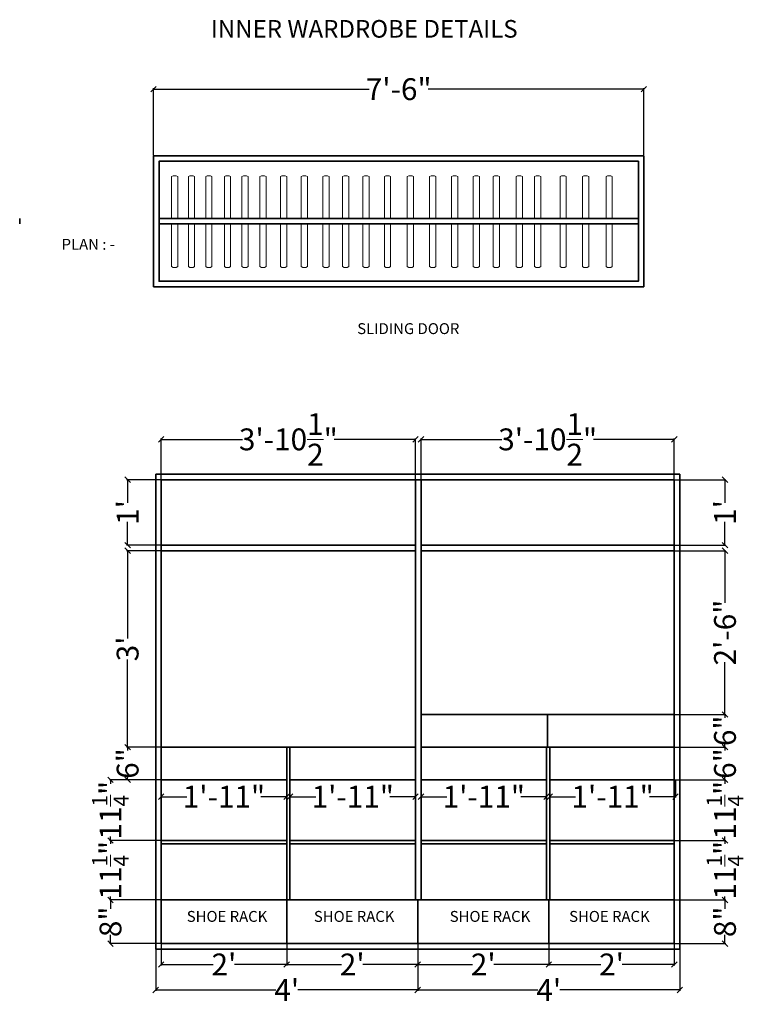
# Model space of a CAD drawing. Units: inches. Extents: x 314 to 446, y 231 to 411.
import ezdxf

# ---------------------------------------------------------------- set-up
doc = ezdxf.new("R2010")
doc.units = ezdxf.units.IN
doc.header["$MEASUREMENT"] = 0
for name, color, linetype, lineweight in [('A-ANNO-DIMS', 2, 'Continuous', 18), ('A-ANNO-TEXT', 7, 'Continuous', 25), ('A-FURN', 7, 'Continuous', 35), ('A-FURN-HANG', 8, 'Continuous', 18)]:
    doc.layers.add(name, color=color, linetype=linetype, lineweight=lineweight)
doc.styles.get("Standard").update_dxf_attribs({"font": 'arial.ttf'})
doc.dimstyles.get("Standard").update_dxf_attribs({"dimtxt": 4, "dimasz": 1, "dimexe": 0.18, "dimexo": 0.0625, "dimgap": 0.09, "dimtad": 0, "dimdec": 1, "dimzin": 0, "dimdsep": 46, "dimlunit": 4, "dimtxsty": 'Standard', "dimblk": 'OBLIQUE', "dimcen": 0.09, "dimadec": 0, "dimazin": 0, "dimtfac": 1, "dimtdec": 1, "dimtofl": 0, "dimtmove": 0, "dimatfit": 3, "dimldrblk": 'OBLIQUE', "dimfxl": 1, "dimtolj": 1, "dimtzin": 0, "dimarcsym": 1})

# ---------------------------------------------------------------- blocks, each defined once
blk = doc.blocks.new('_Oblique')
at = {"color": 0, "linetype": 'ByBlock', "lineweight": -2}
blk.add_line((-0.5, -0.5), (0.5, 0.5), dxfattribs=at)
blk = doc.blocks.new('*D2')
at = {"layer": 'A-ANNO-DIMS', "color": 0, "lineweight": -2, "transparency": 16777216}
for p, q in [((338.41, 386.23), (338.41, 398.53)), ((338.41, 398.35), (377.92, 398.35)), ((428.21, 398.35), (388.7, 398.35)), ((428.21, 386.23), (428.21, 398.53))]:
    blk.add_line(p, q, dxfattribs=at)
at = {"layer": 'Defpoints', "color": 0, "transparency": 16777216}
for p in [(428.21, 398.35), (338.41, 386.16), (428.21, 386.16)]:
    blk.add_point(p, dxfattribs=at)
at = {"layer": 'A-ANNO-DIMS', "color": 0, "lineweight": -2, "transparency": 16777216, "rotation": 180}
blk.add_blockref('_Oblique', (338.41, 398.35), dxfattribs=at)
at = {"layer": 'A-ANNO-DIMS', "color": 0, "lineweight": -2, "transparency": 16777216}
blk.add_blockref('_Oblique', (428.21, 398.35), dxfattribs=at)
at = {"layer": 'A-ANNO-DIMS', "color": 0, "transparency": 16777216, "insert": (383.31, 398.35), "char_height": 4, "width": 10.6003, "attachment_point": 5}
blk.add_mtext('\\A1;7\'-6"', dxfattribs=at)
blk = doc.blocks.new('*D3')
at = {"layer": 'A-ANNO-DIMS', "color": 0, "lineweight": -2, "transparency": 16777216}
for p, q in [((339.8, 271.74), (339.8, 268.55)), ((362.8, 271.74), (362.8, 268.55)), ((339.8, 268.73), (344.52, 268.73)), ((362.8, 268.73), (358.07, 268.73))]:
    blk.add_line(p, q, dxfattribs=at)
at = {"layer": 'Defpoints', "color": 0, "transparency": 16777216}
for p in [(339.8, 271.8), (362.8, 271.8), (339.8, 268.73)]:
    blk.add_point(p, dxfattribs=at)
at = {"layer": 'A-ANNO-DIMS', "color": 0, "lineweight": -2, "transparency": 16777216, "rotation": 180}
blk.add_blockref('_Oblique', (339.8, 268.73), dxfattribs=at)
at = {"layer": 'A-ANNO-DIMS', "color": 0, "lineweight": -2, "transparency": 16777216}
blk.add_blockref('_Oblique', (362.8, 268.73), dxfattribs=at)
at = {"layer": 'A-ANNO-DIMS', "color": 0, "transparency": 16777216, "insert": (351.3, 268.73), "char_height": 4, "attachment_point": 5}
blk.add_mtext('\\A1;1\'-11"', dxfattribs=at)
blk = doc.blocks.new('*D4')
at = {"layer": 'A-ANNO-DIMS', "color": 0, "lineweight": -2, "transparency": 16777216}
for p, q in [((363.4, 271.74), (363.4, 268.55)), ((386.4, 271.74), (386.4, 268.55)), ((363.4, 268.73), (368.12, 268.73)), ((386.4, 268.73), (381.67, 268.73))]:
    blk.add_line(p, q, dxfattribs=at)
at = {"layer": 'Defpoints', "color": 0, "transparency": 16777216}
for p in [(363.4, 271.8), (386.4, 271.8), (386.4, 268.73)]:
    blk.add_point(p, dxfattribs=at)
at = {"layer": 'A-ANNO-DIMS', "color": 0, "lineweight": -2, "transparency": 16777216, "rotation": 180}
blk.add_blockref('_Oblique', (363.4, 268.73), dxfattribs=at)
at = {"layer": 'A-ANNO-DIMS', "color": 0, "lineweight": -2, "transparency": 16777216}
blk.add_blockref('_Oblique', (386.4, 268.73), dxfattribs=at)
at = {"layer": 'A-ANNO-DIMS', "color": 0, "transparency": 16777216, "insert": (374.9, 268.73), "char_height": 4, "attachment_point": 5}
blk.add_mtext('\\A1;1\'-11"', dxfattribs=at)
blk = doc.blocks.new('*D5')
at = {"layer": 'A-ANNO-DIMS', "color": 0, "lineweight": -2, "transparency": 16777216}
for p, q in [((339.8, 241.74), (339.8, 237.81)), ((362.8, 241.74), (362.8, 237.81)), ((339.8, 237.99), (349.33, 237.99)), ((362.8, 237.99), (353.26, 237.99))]:
    blk.add_line(p, q, dxfattribs=at)
at = {"layer": 'Defpoints', "color": 0, "transparency": 16777216}
for p in [(339.8, 241.8), (362.8, 241.8), (362.8, 237.99)]:
    blk.add_point(p, dxfattribs=at)
at = {"layer": 'A-ANNO-DIMS', "color": 0, "lineweight": -2, "transparency": 16777216, "rotation": 180}
blk.add_blockref('_Oblique', (339.8, 237.99), dxfattribs=at)
at = {"layer": 'A-ANNO-DIMS', "color": 0, "lineweight": -2, "transparency": 16777216}
blk.add_blockref('_Oblique', (362.8, 237.99), dxfattribs=at)
at = {"layer": 'A-ANNO-DIMS', "color": 0, "transparency": 16777216, "insert": (351.3, 237.99), "char_height": 4, "attachment_point": 5}
blk.add_mtext("\\A1;2'", dxfattribs=at)
blk = doc.blocks.new('*D6')
at = {"layer": 'A-ANNO-DIMS', "color": 0, "lineweight": -2, "transparency": 16777216}
for p, q in [((362.8, 241.74), (362.8, 237.81)), ((386.8, 241.74), (386.8, 237.81)), ((362.8, 237.99), (372.83, 237.99)), ((386.8, 237.99), (376.76, 237.99))]:
    blk.add_line(p, q, dxfattribs=at)
at = {"layer": 'Defpoints', "color": 0, "transparency": 16777216}
for p in [(362.8, 241.8), (386.8, 241.8), (386.8, 237.99)]:
    blk.add_point(p, dxfattribs=at)
at = {"layer": 'A-ANNO-DIMS', "color": 0, "lineweight": -2, "transparency": 16777216, "rotation": 180}
blk.add_blockref('_Oblique', (362.8, 237.99), dxfattribs=at)
at = {"layer": 'A-ANNO-DIMS', "color": 0, "lineweight": -2, "transparency": 16777216}
blk.add_blockref('_Oblique', (386.8, 237.99), dxfattribs=at)
at = {"layer": 'A-ANNO-DIMS', "color": 0, "transparency": 16777216, "insert": (374.8, 237.99), "char_height": 4, "attachment_point": 5}
blk.add_mtext("\\A1;2'", dxfattribs=at)
blk = doc.blocks.new('*D7')
at = {"layer": 'A-ANNO-DIMS', "color": 0, "lineweight": -2, "transparency": 16777216}
for p, q in [((386.8, 241.74), (386.8, 237.81)), ((410.8, 241.74), (410.8, 237.81)), ((386.8, 237.99), (396.83, 237.99)), ((410.8, 237.99), (400.76, 237.99))]:
    blk.add_line(p, q, dxfattribs=at)
at = {"layer": 'Defpoints', "color": 0, "transparency": 16777216}
for p in [(386.8, 241.8), (410.8, 241.8), (410.8, 237.99)]:
    blk.add_point(p, dxfattribs=at)
at = {"layer": 'A-ANNO-DIMS', "color": 0, "lineweight": -2, "transparency": 16777216, "rotation": 180}
blk.add_blockref('_Oblique', (386.8, 237.99), dxfattribs=at)
at = {"layer": 'A-ANNO-DIMS', "color": 0, "lineweight": -2, "transparency": 16777216}
blk.add_blockref('_Oblique', (410.8, 237.99), dxfattribs=at)
at = {"layer": 'A-ANNO-DIMS', "color": 0, "transparency": 16777216, "insert": (398.8, 237.99), "char_height": 4, "attachment_point": 5}
blk.add_mtext("\\A1;2'", dxfattribs=at)
blk = doc.blocks.new('*D8')
at = {"layer": 'A-ANNO-DIMS', "color": 0, "lineweight": -2, "transparency": 16777216}
for p, q in [((410.8, 241.74), (410.8, 237.81)), ((433.8, 241.74), (433.8, 237.81)), ((410.8, 237.99), (420.33, 237.99)), ((433.8, 237.99), (424.26, 237.99))]:
    blk.add_line(p, q, dxfattribs=at)
at = {"layer": 'Defpoints', "color": 0, "transparency": 16777216}
for p in [(410.8, 241.8), (433.8, 241.8), (410.8, 237.99)]:
    blk.add_point(p, dxfattribs=at)
at = {"layer": 'A-ANNO-DIMS', "color": 0, "lineweight": -2, "transparency": 16777216, "rotation": 180}
blk.add_blockref('_Oblique', (410.8, 237.99), dxfattribs=at)
at = {"layer": 'A-ANNO-DIMS', "color": 0, "lineweight": -2, "transparency": 16777216}
blk.add_blockref('_Oblique', (433.8, 237.99), dxfattribs=at)
at = {"layer": 'A-ANNO-DIMS', "color": 0, "transparency": 16777216, "insert": (422.3, 237.99), "char_height": 4, "attachment_point": 5}
blk.add_mtext("\\A1;2'", dxfattribs=at)
blk = doc.blocks.new('*D9')
at = {"layer": 'A-ANNO-DIMS', "color": 0, "lineweight": -2, "transparency": 16777216}
for p, q in [((338.8, 240.74), (338.8, 233.13)), ((386.8, 240.74), (386.8, 233.13)), ((338.8, 233.31), (360.79, 233.31)), ((386.8, 233.31), (364.81, 233.31))]:
    blk.add_line(p, q, dxfattribs=at)
at = {"layer": 'Defpoints', "color": 0, "transparency": 16777216}
for p in [(338.8, 240.8), (386.8, 240.8), (386.8, 233.31)]:
    blk.add_point(p, dxfattribs=at)
at = {"layer": 'A-ANNO-DIMS', "color": 0, "lineweight": -2, "transparency": 16777216, "rotation": 180}
blk.add_blockref('_Oblique', (338.8, 233.31), dxfattribs=at)
at = {"layer": 'A-ANNO-DIMS', "color": 0, "lineweight": -2, "transparency": 16777216}
blk.add_blockref('_Oblique', (386.8, 233.31), dxfattribs=at)
at = {"layer": 'A-ANNO-DIMS', "color": 0, "transparency": 16777216, "insert": (362.8, 233.31), "char_height": 4, "attachment_point": 5}
blk.add_mtext("\\A1;4'", dxfattribs=at)
blk = doc.blocks.new('*D10')
at = {"layer": 'A-ANNO-DIMS', "color": 0, "lineweight": -2, "transparency": 16777216}
for p, q in [((386.8, 240.74), (386.8, 233.13)), ((434.8, 240.74), (434.8, 233.13)), ((386.8, 233.31), (408.79, 233.31)), ((434.8, 233.31), (412.81, 233.31))]:
    blk.add_line(p, q, dxfattribs=at)
at = {"layer": 'Defpoints', "color": 0, "transparency": 16777216}
for p in [(386.8, 240.8), (434.8, 240.8), (434.8, 233.31)]:
    blk.add_point(p, dxfattribs=at)
at = {"layer": 'A-ANNO-DIMS', "color": 0, "lineweight": -2, "transparency": 16777216, "rotation": 180}
blk.add_blockref('_Oblique', (386.8, 233.31), dxfattribs=at)
at = {"layer": 'A-ANNO-DIMS', "color": 0, "lineweight": -2, "transparency": 16777216}
blk.add_blockref('_Oblique', (434.8, 233.31), dxfattribs=at)
at = {"layer": 'A-ANNO-DIMS', "color": 0, "transparency": 16777216, "insert": (410.8, 233.31), "char_height": 4, "attachment_point": 5}
blk.add_mtext("\\A1;4'", dxfattribs=at)
blk = doc.blocks.new('*D11')
at = {"layer": 'A-ANNO-DIMS', "color": 0, "lineweight": -2, "transparency": 16777216}
for p, q in [((387.4, 271.74), (387.4, 268.55)), ((410.4, 271.74), (410.4, 268.55)), ((387.4, 268.73), (392.12, 268.73)), ((410.4, 268.73), (405.67, 268.73))]:
    blk.add_line(p, q, dxfattribs=at)
at = {"layer": 'Defpoints', "color": 0, "transparency": 16777216}
for p in [(387.4, 271.8), (410.4, 271.8), (387.4, 268.73)]:
    blk.add_point(p, dxfattribs=at)
at = {"layer": 'A-ANNO-DIMS', "color": 0, "lineweight": -2, "transparency": 16777216, "rotation": 180}
blk.add_blockref('_Oblique', (387.4, 268.73), dxfattribs=at)
at = {"layer": 'A-ANNO-DIMS', "color": 0, "lineweight": -2, "transparency": 16777216}
blk.add_blockref('_Oblique', (410.4, 268.73), dxfattribs=at)
at = {"layer": 'A-ANNO-DIMS', "color": 0, "transparency": 16777216, "insert": (398.9, 268.73), "char_height": 4, "attachment_point": 5}
blk.add_mtext('\\A1;1\'-11"', dxfattribs=at)
blk = doc.blocks.new('*D12')
at = {"layer": 'A-ANNO-DIMS', "color": 0, "lineweight": -2, "transparency": 16777216}
for p, q in [((411, 271.74), (411, 268.55)), ((434, 271.74), (434, 268.55)), ((411, 268.73), (415.72, 268.73)), ((434, 268.73), (429.27, 268.73))]:
    blk.add_line(p, q, dxfattribs=at)
at = {"layer": 'Defpoints', "color": 0, "transparency": 16777216}
for p in [(411, 271.8), (434, 271.8), (434, 268.73)]:
    blk.add_point(p, dxfattribs=at)
at = {"layer": 'A-ANNO-DIMS', "color": 0, "lineweight": -2, "transparency": 16777216, "rotation": 180}
blk.add_blockref('_Oblique', (411, 268.73), dxfattribs=at)
at = {"layer": 'A-ANNO-DIMS', "color": 0, "lineweight": -2, "transparency": 16777216}
blk.add_blockref('_Oblique', (434, 268.73), dxfattribs=at)
at = {"layer": 'A-ANNO-DIMS', "color": 0, "transparency": 16777216, "insert": (422.5, 268.73), "char_height": 4, "attachment_point": 5}
blk.add_mtext('\\A1;1\'-11"', dxfattribs=at)
blk = doc.blocks.new('*D13')
at = {"layer": 'A-ANNO-DIMS', "color": 0, "lineweight": -2, "transparency": 16777216}
for p, q in [((339.8, 326.86), (339.8, 334.37)), ((339.8, 334.19), (354.68, 334.19)), ((386.4, 334.19), (371.51, 334.19)), ((386.4, 326.86), (386.4, 334.37))]:
    blk.add_line(p, q, dxfattribs=at)
at = {"layer": 'Defpoints', "color": 0, "transparency": 16777216}
for p in [(386.4, 334.19), (339.8, 326.8), (386.4, 326.8)]:
    blk.add_point(p, dxfattribs=at)
at = {"layer": 'A-ANNO-DIMS', "color": 0, "lineweight": -2, "transparency": 16777216, "rotation": 180}
blk.add_blockref('_Oblique', (339.8, 334.19), dxfattribs=at)
at = {"layer": 'A-ANNO-DIMS', "color": 0, "lineweight": -2, "transparency": 16777216}
blk.add_blockref('_Oblique', (386.4, 334.19), dxfattribs=at)
at = {"layer": 'A-ANNO-DIMS', "color": 0, "transparency": 16777216, "insert": (363.1, 334.19), "char_height": 4, "attachment_point": 5}
blk.add_mtext('\\A1;3\'-10{\\H1x;\\S1/2;}"', dxfattribs=at)
blk = doc.blocks.new('*D14')
at = {"layer": 'A-ANNO-DIMS', "color": 0, "lineweight": -2, "transparency": 16777216}
for p, q in [((387.4, 326.86), (387.4, 334.37)), ((387.4, 334.19), (402.18, 334.19)), ((433.8, 334.19), (419.01, 334.19)), ((433.8, 326.86), (433.8, 334.37))]:
    blk.add_line(p, q, dxfattribs=at)
at = {"layer": 'Defpoints', "color": 0, "transparency": 16777216}
for p in [(433.8, 334.19), (387.4, 326.8), (433.8, 326.8)]:
    blk.add_point(p, dxfattribs=at)
at = {"layer": 'A-ANNO-DIMS', "color": 0, "lineweight": -2, "transparency": 16777216, "rotation": 180}
blk.add_blockref('_Oblique', (387.4, 334.19), dxfattribs=at)
at = {"layer": 'A-ANNO-DIMS', "color": 0, "lineweight": -2, "transparency": 16777216}
blk.add_blockref('_Oblique', (433.8, 334.19), dxfattribs=at)
at = {"layer": 'A-ANNO-DIMS', "color": 0, "transparency": 16777216, "insert": (410.6, 334.19), "char_height": 4, "attachment_point": 5}
blk.add_mtext('\\A1;3\'-10{\\H1x;\\S1/2;}"', dxfattribs=at)
blk = doc.blocks.new('*D15')
at = {"layer": 'A-ANNO-DIMS', "color": 0, "lineweight": -2, "transparency": 16777216}
for p, q in [((433.86, 326.8), (443.26, 326.8)), ((443.08, 326.8), (443.08, 322.54)), ((443.08, 314.8), (443.08, 319.06)), ((433.86, 314.8), (443.26, 314.8))]:
    blk.add_line(p, q, dxfattribs=at)
at = {"layer": 'Defpoints', "color": 0, "transparency": 16777216}
for p in [(433.8, 326.8), (433.8, 314.8), (443.08, 314.8)]:
    blk.add_point(p, dxfattribs=at)
at = {"layer": 'A-ANNO-DIMS', "color": 0, "lineweight": -2, "transparency": 16777216}
for p, rotation in [((443.08, 326.8), 90), ((443.08, 314.8), 270)]:
    blk.add_blockref('_Oblique', p, dxfattribs=dict(at, rotation=rotation))
at = {"layer": 'A-ANNO-DIMS', "color": 0, "transparency": 16777216, "insert": (443.08, 320.8), "char_height": 4, "attachment_point": 5, "rotation": 90}
blk.add_mtext("\\A1;1'", dxfattribs=at)
blk = doc.blocks.new('*D16')
at = {"layer": 'A-ANNO-DIMS', "color": 0, "lineweight": -2, "transparency": 16777216}
for p, q in [((433.86, 313.8), (443.26, 313.8)), ((443.08, 313.8), (443.08, 304.24)), ((443.08, 283.8), (443.08, 293.36)), ((433.86, 283.8), (443.26, 283.8))]:
    blk.add_line(p, q, dxfattribs=at)
at = {"layer": 'Defpoints', "color": 0, "transparency": 16777216}
for p in [(433.8, 313.8), (433.8, 283.8), (443.08, 283.8)]:
    blk.add_point(p, dxfattribs=at)
at = {"layer": 'A-ANNO-DIMS', "color": 0, "lineweight": -2, "transparency": 16777216}
for p, rotation in [((443.08, 313.8), 90), ((443.08, 283.8), 270)]:
    blk.add_blockref('_Oblique', p, dxfattribs=dict(at, rotation=rotation))
at = {"layer": 'A-ANNO-DIMS', "color": 0, "transparency": 16777216, "insert": (443.08, 298.8), "char_height": 4, "attachment_point": 5, "rotation": 90}
blk.add_mtext('\\A1;2\'-6"', dxfattribs=at)
blk = doc.blocks.new('*D17')
at = {"layer": 'A-ANNO-DIMS', "color": 0, "lineweight": -2, "transparency": 16777216}
for p, q in [((433.86, 283.8), (443.26, 283.8)), ((443.08, 283.8), (443.08, 283.2)), ((443.08, 277.8), (443.08, 278.4)), ((433.86, 277.8), (443.26, 277.8))]:
    blk.add_line(p, q, dxfattribs=at)
at = {"layer": 'Defpoints', "color": 0, "transparency": 16777216}
for p in [(433.8, 283.8), (433.8, 277.8), (443.08, 277.8)]:
    blk.add_point(p, dxfattribs=at)
at = {"layer": 'A-ANNO-DIMS', "color": 0, "lineweight": -2, "transparency": 16777216}
for p, rotation in [((443.08, 283.8), 90), ((443.08, 277.8), 270)]:
    blk.add_blockref('_Oblique', p, dxfattribs=dict(at, rotation=rotation))
at = {"layer": 'A-ANNO-DIMS', "color": 0, "transparency": 16777216, "insert": (443.08, 280.8), "char_height": 4, "attachment_point": 5, "rotation": 90}
blk.add_mtext('\\A1;6"', dxfattribs=at)
blk = doc.blocks.new('*D18')
at = {"layer": 'A-ANNO-DIMS', "color": 0, "lineweight": -2, "transparency": 16777216}
for p, q in [((433.86, 277.8), (443.26, 277.8)), ((443.08, 277.8), (443.08, 277.2)), ((443.08, 271.8), (443.08, 272.4)), ((433.86, 271.8), (443.26, 271.8))]:
    blk.add_line(p, q, dxfattribs=at)
at = {"layer": 'Defpoints', "color": 0, "transparency": 16777216}
for p in [(433.8, 277.8), (433.8, 271.8), (443.08, 271.8)]:
    blk.add_point(p, dxfattribs=at)
at = {"layer": 'A-ANNO-DIMS', "color": 0, "lineweight": -2, "transparency": 16777216}
for p, rotation in [((443.08, 277.8), 90), ((443.08, 271.8), 270)]:
    blk.add_blockref('_Oblique', p, dxfattribs=dict(at, rotation=rotation))
at = {"layer": 'A-ANNO-DIMS', "color": 0, "transparency": 16777216, "insert": (443.08, 274.8), "char_height": 4, "attachment_point": 5, "rotation": 90}
blk.add_mtext('\\A1;6"', dxfattribs=at)
blk = doc.blocks.new('*D19')
at = {"layer": 'A-ANNO-DIMS', "color": 0, "lineweight": -2, "transparency": 16777216}
for p, q in [((433.86, 271.8), (443.26, 271.8)), ((443.08, 271.8), (443.08, 271.07)), ((433.86, 260.7), (443.26, 260.7)), ((443.08, 260.7), (443.08, 261.44))]:
    blk.add_line(p, q, dxfattribs=at)
at = {"layer": 'Defpoints', "color": 0, "transparency": 16777216}
for p in [(433.8, 271.8), (433.8, 260.7), (443.08, 260.7)]:
    blk.add_point(p, dxfattribs=at)
at = {"layer": 'A-ANNO-DIMS', "color": 0, "lineweight": -2, "transparency": 16777216}
for p, rotation in [((443.08, 271.8), 90), ((443.08, 260.7), 270)]:
    blk.add_blockref('_Oblique', p, dxfattribs=dict(at, rotation=rotation))
at = {"layer": 'A-ANNO-DIMS', "color": 0, "transparency": 16777216, "insert": (443.08, 266.25), "char_height": 4, "attachment_point": 5, "rotation": 90}
blk.add_mtext('\\A1;11{\\H0.7x;\\S1/4;}"', dxfattribs=at)
blk = doc.blocks.new('*D20')
at = {"layer": 'A-ANNO-DIMS', "color": 0, "lineweight": -2, "transparency": 16777216}
for p, q in [((433.86, 260.7), (443.26, 260.7)), ((443.08, 260.7), (443.08, 260.07)), ((433.86, 249.8), (443.26, 249.8)), ((443.08, 249.8), (443.08, 250.44))]:
    blk.add_line(p, q, dxfattribs=at)
at = {"layer": 'Defpoints', "color": 0, "transparency": 16777216}
for p in [(433.8, 260.7), (433.8, 249.8), (443.08, 249.8)]:
    blk.add_point(p, dxfattribs=at)
at = {"layer": 'A-ANNO-DIMS', "color": 0, "lineweight": -2, "transparency": 16777216}
for p, rotation in [((443.08, 260.7), 90), ((443.08, 249.8), 270)]:
    blk.add_blockref('_Oblique', p, dxfattribs=dict(at, rotation=rotation))
at = {"layer": 'A-ANNO-DIMS', "color": 0, "transparency": 16777216, "insert": (443.08, 255.25), "char_height": 4, "attachment_point": 5, "rotation": 90}
blk.add_mtext('\\A1;11{\\H0.7x;\\S1/4;}"', dxfattribs=at)
blk = doc.blocks.new('*D21')
at = {"layer": 'A-ANNO-DIMS', "color": 0, "lineweight": -2, "transparency": 16777216}
for p, q in [((433.86, 249.8), (443.26, 249.8)), ((443.08, 249.8), (443.08, 248.19)), ((433.86, 241.8), (443.26, 241.8)), ((443.08, 241.8), (443.08, 243.41))]:
    blk.add_line(p, q, dxfattribs=at)
at = {"layer": 'Defpoints', "color": 0, "transparency": 16777216}
for p in [(433.8, 249.8), (433.8, 241.8), (443.08, 241.8)]:
    blk.add_point(p, dxfattribs=at)
at = {"layer": 'A-ANNO-DIMS', "color": 0, "lineweight": -2, "transparency": 16777216}
for p, rotation in [((443.08, 249.8), 90), ((443.08, 241.8), 270)]:
    blk.add_blockref('_Oblique', p, dxfattribs=dict(at, rotation=rotation))
at = {"layer": 'A-ANNO-DIMS', "color": 0, "transparency": 16777216, "insert": (443.08, 245.8), "char_height": 4, "attachment_point": 5, "rotation": 90}
blk.add_mtext('\\A1;8"', dxfattribs=at)
blk = doc.blocks.new('*D22')
at = {"layer": 'A-ANNO-DIMS', "color": 0, "lineweight": -2, "transparency": 16777216}
for p, q in [((339.73, 313.8), (333.48, 313.8)), ((333.66, 313.8), (333.66, 297.73)), ((333.66, 277.8), (333.66, 293.87)), ((339.73, 277.8), (333.48, 277.8))]:
    blk.add_line(p, q, dxfattribs=at)
at = {"layer": 'Defpoints', "color": 0, "transparency": 16777216}
for p in [(339.8, 313.8), (333.66, 277.8), (339.8, 277.8)]:
    blk.add_point(p, dxfattribs=at)
at = {"layer": 'A-ANNO-DIMS', "color": 0, "lineweight": -2, "transparency": 16777216}
for p, rotation in [((333.66, 313.8), 90), ((333.66, 277.8), 270)]:
    blk.add_blockref('_Oblique', p, dxfattribs=dict(at, rotation=rotation))
at = {"layer": 'A-ANNO-DIMS', "color": 0, "transparency": 16777216, "insert": (333.66, 295.8), "char_height": 4, "attachment_point": 5, "rotation": 90}
blk.add_mtext("\\A1;3'", dxfattribs=at)
blk = doc.blocks.new('*D23')
at = {"layer": 'A-ANNO-DIMS', "color": 0, "lineweight": -2, "transparency": 16777216}
for p, q in [((339.73, 326.8), (333.48, 326.8)), ((333.66, 326.8), (333.66, 322.54)), ((333.66, 314.8), (333.66, 319.06)), ((339.73, 314.8), (333.48, 314.8))]:
    blk.add_line(p, q, dxfattribs=at)
at = {"layer": 'Defpoints', "color": 0, "transparency": 16777216}
for p in [(339.8, 326.8), (333.66, 314.8), (339.8, 314.8)]:
    blk.add_point(p, dxfattribs=at)
at = {"layer": 'A-ANNO-DIMS', "color": 0, "lineweight": -2, "transparency": 16777216}
for p, rotation in [((333.66, 326.8), 90), ((333.66, 314.8), 270)]:
    blk.add_blockref('_Oblique', p, dxfattribs=dict(at, rotation=rotation))
at = {"layer": 'A-ANNO-DIMS', "color": 0, "transparency": 16777216, "insert": (333.66, 320.8), "char_height": 4, "attachment_point": 5, "rotation": 90}
blk.add_mtext("\\A1;1'", dxfattribs=at)
blk = doc.blocks.new('*D24')
at = {"layer": 'A-ANNO-DIMS', "color": 0, "lineweight": -2, "transparency": 16777216}
for p, q in [((339.73, 277.8), (333.48, 277.8)), ((333.66, 277.8), (333.66, 277.2)), ((333.66, 271.8), (333.66, 272.4)), ((339.73, 271.8), (333.48, 271.8))]:
    blk.add_line(p, q, dxfattribs=at)
at = {"layer": 'Defpoints', "color": 0, "transparency": 16777216}
for p in [(339.8, 277.8), (333.66, 271.8), (339.8, 271.8)]:
    blk.add_point(p, dxfattribs=at)
at = {"layer": 'A-ANNO-DIMS', "color": 0, "lineweight": -2, "transparency": 16777216}
for p, rotation in [((333.66, 277.8), 90), ((333.66, 271.8), 270)]:
    blk.add_blockref('_Oblique', p, dxfattribs=dict(at, rotation=rotation))
at = {"layer": 'A-ANNO-DIMS', "color": 0, "transparency": 16777216, "insert": (333.66, 274.8), "char_height": 4, "attachment_point": 5, "rotation": 90}
blk.add_mtext('\\A1;6"', dxfattribs=at)
blk = doc.blocks.new('*D25')
at = {"layer": 'A-ANNO-DIMS', "color": 0, "lineweight": -2, "transparency": 16777216}
for p, q in [((339.73, 271.8), (330.34, 271.8)), ((330.52, 271.8), (330.52, 271.07)), ((339.73, 260.7), (330.34, 260.7)), ((330.52, 260.7), (330.52, 261.44))]:
    blk.add_line(p, q, dxfattribs=at)
at = {"layer": 'Defpoints', "color": 0, "transparency": 16777216}
for p in [(339.8, 271.8), (330.52, 260.7), (339.8, 260.7)]:
    blk.add_point(p, dxfattribs=at)
at = {"layer": 'A-ANNO-DIMS', "color": 0, "lineweight": -2, "transparency": 16777216}
for p, rotation in [((330.52, 271.8), 90), ((330.52, 260.7), 270)]:
    blk.add_blockref('_Oblique', p, dxfattribs=dict(at, rotation=rotation))
at = {"layer": 'A-ANNO-DIMS', "color": 0, "transparency": 16777216, "insert": (330.52, 266.25), "char_height": 4, "attachment_point": 5, "rotation": 90}
blk.add_mtext('\\A1;11{\\H0.7x;\\S1/4;}"', dxfattribs=at)
blk = doc.blocks.new('*D26')
at = {"layer": 'A-ANNO-DIMS', "color": 0, "lineweight": -2, "transparency": 16777216}
for p, q in [((339.73, 260.7), (330.34, 260.7)), ((330.52, 260.7), (330.52, 260.07)), ((339.73, 249.8), (330.34, 249.8)), ((330.52, 249.8), (330.52, 250.44))]:
    blk.add_line(p, q, dxfattribs=at)
at = {"layer": 'Defpoints', "color": 0, "transparency": 16777216}
for p in [(339.8, 260.7), (330.52, 249.8), (339.8, 249.8)]:
    blk.add_point(p, dxfattribs=at)
at = {"layer": 'A-ANNO-DIMS', "color": 0, "lineweight": -2, "transparency": 16777216}
for p, rotation in [((330.52, 260.7), 90), ((330.52, 249.8), 270)]:
    blk.add_blockref('_Oblique', p, dxfattribs=dict(at, rotation=rotation))
at = {"layer": 'A-ANNO-DIMS', "color": 0, "transparency": 16777216, "insert": (330.52, 255.25), "char_height": 4, "attachment_point": 5, "rotation": 90}
blk.add_mtext('\\A1;11{\\H0.7x;\\S1/4;}"', dxfattribs=at)
blk = doc.blocks.new('*D27')
at = {"layer": 'A-ANNO-DIMS', "color": 0, "lineweight": -2, "transparency": 16777216}
for p, q in [((339.73, 249.8), (330.34, 249.8)), ((330.52, 249.8), (330.52, 248.19)), ((339.73, 241.8), (330.34, 241.8)), ((330.52, 241.8), (330.52, 243.41))]:
    blk.add_line(p, q, dxfattribs=at)
at = {"layer": 'Defpoints', "color": 0, "transparency": 16777216}
for p in [(339.8, 249.8), (330.52, 241.8), (339.8, 241.8)]:
    blk.add_point(p, dxfattribs=at)
at = {"layer": 'A-ANNO-DIMS', "color": 0, "lineweight": -2, "transparency": 16777216}
for p, rotation in [((330.52, 249.8), 90), ((330.52, 241.8), 270)]:
    blk.add_blockref('_Oblique', p, dxfattribs=dict(at, rotation=rotation))
at = {"layer": 'A-ANNO-DIMS', "color": 0, "transparency": 16777216, "insert": (330.52, 245.8), "char_height": 4, "attachment_point": 5, "rotation": 90}
blk.add_mtext('\\A1;8"', dxfattribs=at)
blk = doc.blocks.new('HANGER-A')
for points in [[(0, 0), (0, 7.66)], [(1.14, 7.66), (1.14, 0)]]:
    blk.add_lwpolyline(points)
blk.add_arc((0.57, 6.82), 1.01, 55.7557, 124.2443)
blk = doc.blocks.new('HANGER-B')
for points in [[(0, 0.18), (0, 0.18), (0, 8.01)], [(1.14, 8.01), (1.14, 0.18)]]:
    blk.add_lwpolyline(points)
blk.add_arc((0.57, 1.01), 1.01, 235.7557, 304.2443)
blk = doc.blocks.new('HANGER-C')
for points in [[(0, 0.18), (0, 8.01)], [(1.14, 8.01), (1.14, 0.18)]]:
    blk.add_lwpolyline(points)
blk.add_arc((0.57, 1.01), 1.01, 235.7557, 304.2443)

msp = doc.modelspace()

# ---------------------------------------------------------------- linework, layer by layer
at = {"layer": 'A-FURN'}
for p, q in [((313.89, 373.66), (313.89, 374.66)), ((339.41, 374.66), (427.21, 374.66)), ((427.21, 373.66), (339.41, 373.66)), ((338.8, 240.8), (338.8, 327.8)), ((338.8, 327.8), (434.8, 327.8)), ((339.8, 241.8), (339.8, 326.8)), ((339.8, 326.8), (433.8, 326.8)), ((386.4, 326.8), (386.4, 249.8)), ((387.4, 249.8), (387.4, 326.8)), ((433.8, 326.8), (433.8, 241.8)), ((434.8, 327.8), (434.8, 240.8)), ((339.8, 314.8), (386.4, 314.8)), ((387.4, 314.8), (433.8, 314.8)), ((339.8, 313.8), (386.4, 313.8)), ((387.4, 313.8), (433.8, 313.8)), ((387.4, 283.8), (433.8, 283.8)), ((410.6, 283.8), (410.6, 277.8)), ((339.8, 277.8), (386.4, 277.8)), ((362.8, 277.8), (362.8, 249.8)), ((363.4, 249.8), (363.4, 277.8)), ((387.4, 277.8), (433.8, 277.8)), ((410.4, 277.8), (410.4, 249.8)), ((411, 249.8), (411, 277.8)), ((339.8, 271.8), (362.8, 271.8)), ((363.4, 271.8), (386.4, 271.8)), ((387.4, 271.8), (410.4, 271.8)), ((411, 271.8), (433.8, 271.8)), ((339.8, 260.7), (362.8, 260.7)), ((339.8, 260.1), (362.8, 260.1)), ((363.4, 260.7), (386.4, 260.7)), ((363.4, 260.1), (386.4, 260.1)), ((387.4, 260.7), (410.4, 260.7)), ((387.4, 260.1), (410.4, 260.1)), ((411, 260.7), (433.8, 260.7)), ((411, 260.1), (433.8, 260.1)), ((433.8, 249.8), (339.8, 249.8)), ((362.8, 249.8), (362.8, 241.8)), ((386.8, 249.8), (386.8, 241.8)), ((410.8, 249.8), (410.8, 241.8)), ((433.8, 241.8), (339.8, 241.8)), ((434.8, 240.8), (338.8, 240.8))]:
    msp.add_line(p, q, dxfattribs=at)
for points in [[(428.21, 386.16), (428.21, 362.16), (338.41, 362.16), (338.41, 386.16)], [(427.21, 385.16), (427.21, 363.16), (339.41, 363.16), (339.41, 385.16)]]:
    msp.add_lwpolyline(points, close=True, dxfattribs=at)

# ---------------------------------------------------------------- block references
at = {"layer": 'A-FURN-HANG'}
for name, p in [('HANGER-A', (341.71, 374.67)), ('HANGER-A', (344.8, 374.67)), ('HANGER-A', (347.97, 374.67)), ('HANGER-A', (351.38, 374.67)), ('HANGER-A', (354.58, 374.67)), ('HANGER-A', (357.89, 374.67)), ('HANGER-A', (361.66, 374.67)), ('HANGER-A', (365.45, 374.67)), ('HANGER-A', (369.43, 374.67)), ('HANGER-A', (373.02, 374.67)), ('HANGER-A', (376.75, 374.67)), ('HANGER-A', (380.7, 374.67)), ('HANGER-A', (384.89, 374.67)), ('HANGER-A', (388.98, 374.67)), ('HANGER-A', (393, 374.67)), ('HANGER-A', (396.97, 374.67)), ('HANGER-A', (400.61, 374.67)), ('HANGER-A', (404.83, 374.67)), ('HANGER-A', (408.2, 374.67)), ('HANGER-A', (412.88, 374.67)), ('HANGER-A', (416.98, 374.67)), ('HANGER-A', (421.29, 374.67)), ('HANGER-B', (341.71, 365.66)), ('HANGER-C', (344.8, 365.66)), ('HANGER-B', (347.97, 365.66)), ('HANGER-B', (351.38, 365.66)), ('HANGER-B', (354.58, 365.66)), ('HANGER-B', (357.89, 365.66)), ('HANGER-B', (361.66, 365.66)), ('HANGER-B', (365.45, 365.66)), ('HANGER-B', (369.43, 365.66)), ('HANGER-B', (373.02, 365.66)), ('HANGER-B', (376.75, 365.66)), ('HANGER-B', (380.7, 365.66)), ('HANGER-B', (384.89, 365.66)), ('HANGER-B', (388.98, 365.66)), ('HANGER-B', (393, 365.66)), ('HANGER-B', (396.97, 365.66)), ('HANGER-B', (400.61, 365.66)), ('HANGER-B', (404.83, 365.66)), ('HANGER-B', (408.2, 365.66)), ('HANGER-C', (412.88, 365.66)), ('HANGER-B', (416.98, 365.66)), ('HANGER-B', (421.29, 365.66))]:
    msp.add_blockref(name, p, dxfattribs=at)

# ---------------------------------------------------------------- texts
at = {"layer": 'A-ANNO-TEXT', "attachment_point": 1}
for s, width, gutter_width, insert, char_height in [('\\pxqc;INNER WARDROBE DETAILS', 100.5871, 16.14, (326.7, 411.02), 3.2289), ('\\pxqc;PLAN : - ', 32.0787, 10, (310.41, 370.93), 2), ('\\pxqc;SLIDING DOOR', 62.0899, 10, (354.03, 355.48), 2), ('\\pxqc;SHOE RACK', 18.2941, 10, (342.72, 247.79), 2), ('\\pxqc;SHOE RACK', 18.2941, 10, (366.01, 247.79), 2), ('\\pxqc;SHOE RACK', 18.2941, 10, (390.89, 247.79), 2), ('\\pxqc;SHOE RACK', 18.2941, 10, (412.76, 247.79), 2)]:
    msp.add_mtext_dynamic_manual_height_columns(s, width=width, gutter_width=gutter_width, heights=[0], dxfattribs=dict(at, insert=insert, char_height=char_height))

# ---------------------------------------------------------------- dimensions: what is measured, and where the dimension line sits
at = {"layer": 'A-ANNO-DIMS'}
for base, p1, p2, picture, middle in [((428.21, 398.35), (338.41, 386.16), (428.21, 386.16), '*D2', (383.31, 398.35)), ((386.4, 334.19), (339.8, 326.8), (386.4, 326.8), '*D13', (363.1, 334.19)), ((433.8, 334.19), (387.4, 326.8), (433.8, 326.8), '*D14', (410.6, 334.19)), ((339.8, 268.73), (362.8, 271.8), (339.8, 271.8), '*D3', (351.3, 268.73)), ((386.4, 268.73), (363.4, 271.8), (386.4, 271.8), '*D4', (374.9, 268.73)), ((387.4, 268.73), (410.4, 271.8), (387.4, 271.8), '*D11', (398.9, 268.73)), ((434, 268.73), (411, 271.8), (434, 271.8), '*D12', (422.5, 268.73)), ((386.8, 237.99), (362.8, 241.8), (386.8, 241.8), '*D6', (374.8, 237.99)), ((410.8, 237.99), (386.8, 241.8), (410.8, 241.8), '*D7', (398.8, 237.99)), ((386.8, 233.31), (338.8, 240.8), (386.8, 240.8), '*D9', (362.8, 233.31)), ((434.8, 233.31), (386.8, 240.8), (434.8, 240.8), '*D10', (410.8, 233.31))]:
    dim = msp.add_linear_dim(base=base, p1=p1, p2=p2, dimstyle='Standard', override={"dimclrd": 0, "dimclre": 0, "dimclrt": 0}, dxfattribs=at)
    dim.commit()
    dim.dimension.update_dxf_attribs({"geometry": picture, "text_midpoint": middle})
for base, p1, p2, picture, middle in [((333.66, 314.8), (339.8, 326.8), (339.8, 314.8), '*D23', (333.66, 320.8)), ((443.08, 314.8), (433.8, 326.8), (433.8, 314.8), '*D15', (443.08, 320.8)), ((333.66, 277.8), (339.8, 313.8), (339.8, 277.8), '*D22', (333.66, 295.8)), ((443.08, 283.8), (433.8, 313.8), (433.8, 283.8), '*D16', (443.08, 298.8)), ((443.08, 277.8), (433.8, 283.8), (433.8, 277.8), '*D17', (443.08, 280.8)), ((333.66, 271.8), (339.8, 277.8), (339.8, 271.8), '*D24', (333.66, 274.8)), ((443.08, 271.8), (433.8, 277.8), (433.8, 271.8), '*D18', (443.08, 274.8)), ((330.52, 241.8), (339.8, 249.8), (339.8, 241.8), '*D27', (330.52, 245.8)), ((443.08, 241.8), (433.8, 249.8), (433.8, 241.8), '*D21', (443.08, 245.8))]:
    dim = msp.add_linear_dim(base=base, p1=p1, p2=p2, angle=90, dimstyle='Standard', override={"dimclrd": 0, "dimclre": 0, "dimclrt": 0}, dxfattribs=at)
    dim.commit()
    dim.dimension.update_dxf_attribs({"geometry": picture, "text_midpoint": middle})
for base, p1, p2, picture, middle in [((330.52, 260.7), (339.8, 271.8), (339.8, 260.7), '*D25', (330.52, 266.25)), ((443.08, 260.7), (433.8, 271.8), (433.8, 260.7), '*D19', (443.08, 266.25)), ((330.52, 249.8), (339.8, 260.7), (339.8, 249.8), '*D26', (330.52, 255.25)), ((443.08, 249.8), (433.8, 260.7), (433.8, 249.8), '*D20', (443.08, 255.25))]:
    dim = msp.add_linear_dim(base=base, p1=p1, p2=p2, angle=90, text='11{\\H0.7x;\\S1/4;}"', dimstyle='Standard', override={"dimclrd": 0, "dimclre": 0, "dimclrt": 0}, dxfattribs=at)
    dim.commit()
    dim.dimension.update_dxf_attribs({"geometry": picture, "text_midpoint": middle})
for base, p1, p2, picture, middle in [((362.8, 237.99), (339.8, 241.8), (362.8, 241.8), '*D5', (351.3, 237.99)), ((410.8, 237.99), (433.8, 241.8), (410.8, 241.8), '*D8', (422.3, 237.99))]:
    dim = msp.add_linear_dim(base=base, p1=p1, p2=p2, text="2'", dimstyle='Standard', override={"dimclrd": 0, "dimclre": 0, "dimclrt": 0}, dxfattribs=at)
    dim.commit()
    dim.dimension.update_dxf_attribs({"geometry": picture, "text_midpoint": middle})

doc.saveas('drawing.dxf')
